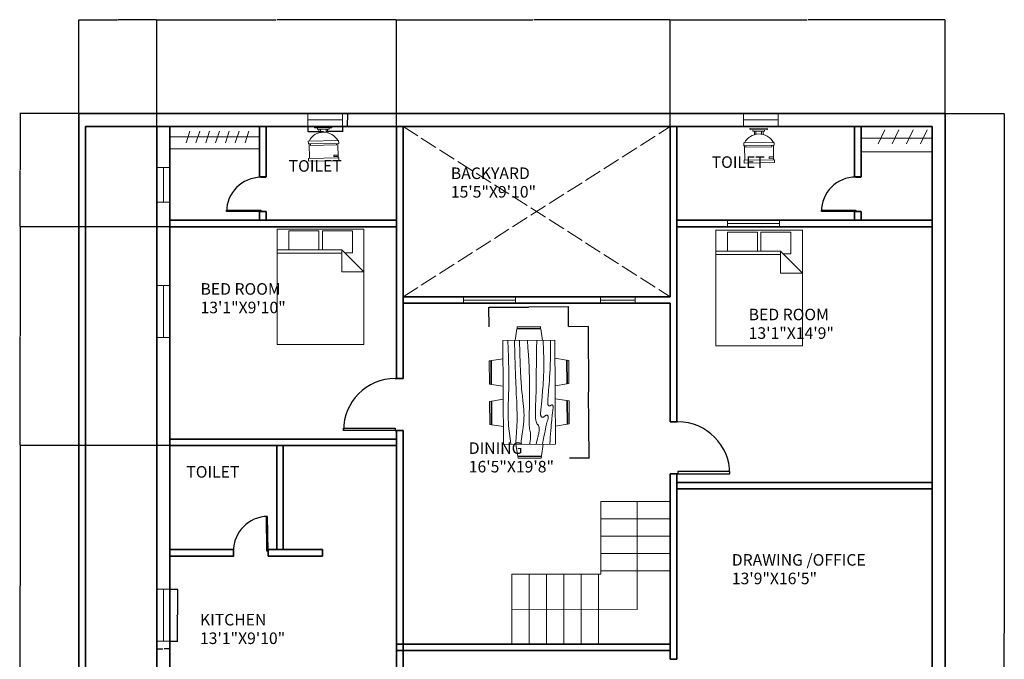
# Model space of a CAD drawing. Units: inches. Extents: x 267 to 949, y 280 to 1117.
# Tile 2 of 2: x 267 to 949, y 674 to 1117. Entities that reach past the tile are written whole.
import ezdxf

# ---------------------------------------------------------------- set-up
doc = ezdxf.new("R2010")
doc.units = ezdxf.units.IN
doc.linetypes.add('ACAD_ISO02W100', pattern=[15, 12, -3])
for name, color, linetype, lineweight in [('A-ANNO-DIMS', 2, 'Continuous', 18), ('A-AREA-IDEN', 5, 'Continuous', 18), ('A-FLOR-FIXT', 3, 'Continuous', 18), ('A-FLOR-OPEN', 3, 'ACAD_ISO02W100', 13), ('A-FURN-FIXD', 3, 'Continuous', 18), ('A-FURN-PATT', 8, 'Continuous', 13), ('DOOR', 1, 'Continuous', 25), ('FUR', 3, 'Continuous', 18), ('STAIR', 4, 'Continuous', 18), ('WALL', 7, 'Continuous', 35), ('WIN', 2, 'Continuous', 20)]:
    doc.layers.add(name, color=color, linetype=linetype, lineweight=lineweight)
doc.styles.get("Standard").update_dxf_attribs({"font": 'arial.ttf'})
doc.dimstyles.get("Standard").update_dxf_attribs({"dimtxt": 0.18, "dimasz": 0.18, "dimexe": 0.18, "dimexo": 0.0625, "dimgap": 0.09, "dimtad": 0, "dimtih": 1, "dimtoh": 1, "dimdec": 4, "dimzin": 0, "dimdsep": 46, "dimtxsty": 'Standard', "dimcen": 0.09, "dimadec": 0, "dimazin": 0, "dimtfac": 1, "dimtdec": 4, "dimtofl": 0, "dimtmove": 0, "dimatfit": 3, "dimfxl": 1, "dimtolj": 1, "dimtzin": 0, "dimarcsym": 0})

# ---------------------------------------------------------------- blocks, each defined once
blk = doc.blocks.new('*U2')
for p, q in [((0, 0), (0, -6)), ((40, 0), (40, -6))]:
    blk.add_line(p, q)
blk.add_lwpolyline([(0, 0), (0, 40), (1.75, 40), (1.75, 0)], close=True)
blk.add_arc((0, 0), 40, 0, 90)
blk = doc.blocks.new('*U3')
for p, q in [((0, 0), (0, 6)), ((40, 0), (40, 6))]:
    blk.add_line(p, q)
blk.add_lwpolyline([(0, 0), (0, -40), (1.75, -40), (1.75, 0)], close=True)
blk.add_arc((0, 0), 40, 270, 360)
blk = doc.blocks.new('*U4')
for p, q in [((0, 0), (0, 6)), ((40, 0), (40, 6))]:
    blk.add_line(p, q)
blk.add_lwpolyline([(0, 0), (0, -40), (1.75, -40), (1.75, 0)], close=True)
blk.add_arc((0, 0), 40, 270, 0)
blk = doc.blocks.new('Bed - Queen')
for p, q in [((0, -80.00003), (0, 0)), ((0, 0), (59.99999, 0)), ((59.99999, 0), (59.99999, -80.00003)), ((7.99999, -1.2), (28.79998, -1.2)), ((7.99999, -14.4), (7.99999, -1.2)), ((28.79998, -1.2), (28.79998, -14.4)), ((31.19999, -1.2), (51.99999, -1.2)), ((31.19999, -14.4), (31.19999, -1.2)), ((51.99999, -1.2), (51.99999, -16.4)), ((0, -14.4), (44.8, -14.4)), ((44.8, -16.8), (0, -16.8)), ((59.99999, -29.6), (44.8, -14.4)), ((44.8, -14.4), (44.8, -29.6)), ((51.99999, -16.4), (46.79936, -16.4)), ((44.8, -29.6), (59.99999, -29.6)), ((59.99999, -80.00003), (0, -80.00003))]:
    blk.add_line(p, q)
blk = doc.blocks.new('Dining Set - 36 x 72 in.')
for p, q in [((-22, 27.5), (-22.1562, 26.50042)), ((-22, 27.5), (-6, 27.5)), ((-5.8437, 26.49966), (-6, 27.5)), ((6, 27.5), (5.8438, 26.50042)), ((6, 27.5), (22, 27.5)), ((22.1563, 26.49966), (22, 27.5)), ((-22.2343, 26.00059), (-23.4847, 17.99762)), ((-22.2304, 26), (-5.7608, 26)), ((-5.8416, 26.5), (-22.1534, 26.5)), ((-4.5152, 17.99762), (-5.7655, 25.99926)), ((5.7657, 26.00059), (4.5153, 17.99762)), ((5.7696, 26), (22.2392, 26)), ((22.1584, 26.5), (5.8466, 26.5)), ((23.4848, 17.99762), (22.2345, 25.99926)), ((36, 18), (-36, 18)), ((-36, 18), (-36, -18)), ((36, -18), (36, 18)), ((-45.5, 8), (-44.5004, 8.15617)), ((-45.5, 8), (-45.5, -8)), ((-44.5, -8.15843), (-44.5, 8.15338)), ((-44.0006, 8.23428), (-35.9976, 9.48474)), ((-44, 8.23041), (-44, -8.23915)), ((44.0006, 8.23428), (35.9976, 9.48474)), ((44, 8.23041), (44, -8.23915)), ((44.5, -8.15843), (44.5, 8.15338)), ((45.5, 8), (44.5005, 8.15617)), ((45.5, 8), (45.5, -8)), ((-44.4997, -8.15631), (-45.5, -8)), ((-35.9976, -9.48476), (-43.9993, -8.2345)), ((35.9976, -9.48476), (43.9993, -8.2345)), ((44.4997, -8.15631), (45.5, -8)), ((-36, -18), (36, -18)), ((-22.2343, -26.0006), (-23.4847, -17.99762)), ((-4.5152, -17.99762), (-5.7655, -25.99928)), ((5.7657, -26.0006), (4.5153, -17.99762)), ((23.4848, -17.99762), (22.2345, -25.99928)), ((-22.2304, -26), (-5.7608, -26)), ((-22, -27.5), (-22.1562, -26.50044)), ((-5.8416, -26.5), (-22.1534, -26.5)), ((-5.8437, -26.49967), (-6, -27.5)), ((5.7696, -26), (22.2392, -26)), ((6, -27.5), (5.8438, -26.50044)), ((22.1584, -26.5), (5.8466, -26.5)), ((22.1563, -26.49967), (22, -27.5)), ((-22, -27.5), (-6, -27.5)), ((6, -27.5), (22, -27.5))]:
    blk.add_line(p, q)
for points in [[(-36, 15), (-31.1772, 14.97754), (-26.8079, 14.91406), (-22.8538, 14.81543), (-19.276, 14.6875), (-16.0362, 14.53613), (-13.0957, 14.36718), (-10.4159, 14.18652), (-7.9583, 14), (-5.6904, 13.81315), (-3.6035, 13.63021), (-1.6954, 13.45508), (0.0365, 13.29166), (1.5945, 13.14388), (2.9811, 13.01562), (4.1988, 12.9108), (5.25, 12.83333), (6.1393, 12.78613), (6.8802, 12.76823), (7.4883, 12.77767), (7.9792, 12.8125), (8.3685, 12.87077), (8.6719, 12.95052), (8.9049, 13.0498), (9.0833, 13.16666), (9.2205, 13.29899), (9.3216, 13.44401), (9.3895, 13.59879), (9.4271, 13.76041), (9.4373, 13.92594), (9.4232, 14.09245), (9.3875, 14.257), (9.3333, 14.41666), (9.2638, 14.56917), (9.1836, 14.71484), (9.0975, 14.85465), (9.0104, 14.98958), (8.9272, 15.1206), (8.8529, 15.2487), (8.7922, 15.37483), (8.75, 15.5), (8.7305, 15.62467), (8.7344, 15.74739), (8.7617, 15.86621), (8.8125, 15.97916), (8.8867, 16.08431), (8.9844, 16.17968), (9.1055, 16.26334), (9.25, 16.33333), (9.4189, 16.38802), (9.6172, 16.42708), (9.8506, 16.45052), (10.125, 16.45833), (10.4463, 16.45052), (10.8203, 16.42708), (11.2529, 16.38802), (11.75, 16.33333), (12.3184, 16.26318), (12.9694, 16.17838), (13.7151, 16.07991), (14.5677, 15.96875), (15.5395, 15.84586), (16.6426, 15.71224), (17.8893, 15.56884), (19.2917, 15.41666), (20.859, 15.25667), (22.5879, 15.08984), (24.4721, 14.91715), (26.5052, 14.73958), (28.6809, 14.5581), (30.9929, 14.3737), (33.4347, 14.18733), (36, 14)], [(-36, 10), (-28.9766, 10.14274), (-23.1725, 10.20442), (-18.4241, 10.19775), (-14.5677, 10.13541), (-11.4399, 10.03011), (-8.877, 9.89453), (-6.7154, 9.74137), (-4.7917, 9.58333), (-2.9698, 9.43082), (-1.2246, 9.28515), (0.4415, 9.14534), (2.026, 9.01041), (3.5266, 8.87939), (4.9408, 8.7513), (6.266, 8.62516), (7.5, 8.5), (8.6411, 8.37549), (9.6914, 8.2539), (10.6538, 8.13818), (11.5312, 8.03125), (12.3267, 7.93603), (13.043, 7.85547), (13.6831, 7.79248), (14.25, 7.75), (14.7471, 7.7303), (15.1797, 7.73307), (15.5537, 7.75732), (15.875, 7.80208), (16.1494, 7.86637), (16.3828, 7.94922), (16.5811, 8.04964), (16.75, 8.16666), (16.8944, 8.29915), (17.0143, 8.44531), (17.1089, 8.60319), (17.1771, 8.77083), (17.218, 8.94629), (17.2305, 9.1276), (17.2137, 9.31282), (17.1667, 9.5), (17.0895, 9.6875), (16.987, 9.875), (16.8649, 10.0625), (16.7292, 10.25), (16.5856, 10.4375), (16.4401, 10.625), (16.2985, 10.8125), (16.1667, 11), (16.05, 11.18733), (15.9518, 11.3737), (15.8752, 11.5581), (15.8229, 11.73958), (15.798, 11.91715), (15.8034, 12.08984), (15.842, 12.25667), (15.9167, 12.41666), (16.0295, 12.56836), (16.1784, 12.70833), (16.3605, 12.83268), (16.5729, 12.9375), (16.8127, 13.01888), (17.0768, 13.07291), (17.3625, 13.0957), (17.6667, 13.08333), (17.9894, 13.03312), (18.3418, 12.94726), (18.7382, 12.82918), (19.1927, 12.68229), (19.7195, 12.51001), (20.3327, 12.31575), (21.0465, 12.10294), (21.875, 11.875), (22.8357, 11.63354), (23.959, 11.37304), (25.2786, 11.08618), (26.8282, 10.76562), (28.6414, 10.40405), (30.752, 9.99414), (33.1936, 9.52856), (36, 9)], [(-36, 5.5), (-30.7157, 5.3348), (-26.069, 5.20963), (-21.9946, 5.11767), (-18.4271, 5.05208), (-15.3009, 5.00602), (-12.5508, 4.97265), (-10.1112, 4.94515), (-7.9167, 4.91666), (-5.909, 4.88167), (-4.0586, 4.83984), (-2.3429, 4.79215), (-0.7396, 4.73958), (0.7739, 4.6831), (2.22, 4.6237), (3.6213, 4.56233), (5, 4.5), (6.373, 4.43782), (7.7344, 4.3776), (9.0723, 4.32129), (10.375, 4.27083), (11.6309, 4.22819), (12.8281, 4.19531), (13.9551, 4.17415), (15, 4.16666), (15.954, 4.17448), (16.819, 4.19791), (17.6001, 4.23698), (18.3021, 4.29166), (18.9299, 4.36198), (19.4883, 4.44791), (19.9823, 4.54948), (20.4167, 4.66666), (20.7969, 4.79899), (21.1302, 4.94401), (21.4245, 5.09879), (21.6875, 5.26041), (21.9271, 5.42594), (22.1511, 5.59245), (22.3672, 5.757), (22.5834, 5.91666), (22.8065, 6.06868), (23.0404, 6.21093), (23.2879, 6.34147), (23.5521, 6.45833), (23.8358, 6.55957), (24.142, 6.64323), (24.4735, 6.70735), (24.8334, 6.75), (25.2235, 6.76969), (25.642, 6.76692), (26.0858, 6.74267), (26.5521, 6.69791), (27.0379, 6.63362), (27.5404, 6.55078), (28.0565, 6.45036), (28.5834, 6.33333), (29.1242, 6.19987), (29.7071, 6.04687), (30.3661, 5.87044), (31.1354, 5.66666), (32.0493, 5.43164), (33.142, 5.16146), (34.4475, 4.85221), (36, 4.5)], [(-36, -1), (-30.7915, -0.6591), (-26.0195, -0.38216), (-21.6519, -0.16284), (-17.6563, 0.00521), (-14.0005, 0.12833), (-10.6523, 0.21289), (-7.5796, 0.26522), (-4.75, 0.29166), (-2.134, 0.29793), (0.2878, 0.28711), (2.5317, 0.26163), (4.6146, 0.22396), (6.5529, 0.17651), (8.3633, 0.12174), (10.0623, 0.06209), (11.6667, 0), (13.1899, -0.06201), (14.6341, -0.1211), (15.9982, -0.17432), (17.2813, -0.21875), (18.4823, -0.25147), (19.6003, -0.26953), (20.6343, -0.27002), (21.5834, -0.25), (22.4481, -0.20768), (23.2357, -0.14584), (23.9549, -0.06836), (24.6146, 0.02083), (25.2235, 0.11784), (25.7904, 0.21875), (26.3241, 0.31966), (26.8334, 0.41666), (27.3265, 0.50618), (27.8099, 0.58593), (28.2894, 0.65397), (28.7709, 0.70833), (29.2601, 0.74707), (29.763, 0.76823), (30.2855, 0.76985), (30.8334, 0.75), (31.4088, 0.70784), (31.9994, 0.64713), (32.589, 0.57275), (33.1615, 0.48958), (33.7008, 0.4025), (34.1908, 0.3164), (34.6153, 0.23616), (34.9584, 0.16666), (35.2099, 0.11165), (35.3848, 0.07031), (35.504, 0.04069), (35.5886, 0.02083), (35.6594, 0.00879), (35.7377, 0.0026), (35.8442, 0.00032), (36, 0)], [(-36, -6.5), (-27.1843, -6.31267), (-20.084, -6.1263), (-14.469, -5.9419), (-10.1094, -5.76042), (-6.7752, -5.58285), (-4.2363, -5.41016), (-2.2629, -5.24333), (-0.625, -5.08334), (0.8708, -4.93099), (2.2715, -4.78646), (3.5872, -4.64974), (4.8281, -4.52084), (6.0046, -4.39974), (7.127, -4.28646), (8.2053, -4.18099), (9.25, -4.08334), (10.2705, -3.99382), (11.2734, -3.91407), (12.2647, -3.84603), (13.25, -3.79167), (14.2354, -3.75293), (15.2266, -3.73177), (16.2295, -3.73015), (17.25, -3.75), (18.2912, -3.79248), (19.3451, -3.85547), (20.4009, -3.93604), (21.4479, -4.03125), (22.4754, -4.13819), (23.4727, -4.25391), (24.4289, -4.37549), (25.3334, -4.5), (26.1785, -4.62492), (26.9694, -4.74935), (27.7145, -4.87281), (28.4219, -4.99479), (29.1, -5.11483), (29.7572, -5.23242), (30.4016, -5.34709), (31.0417, -5.45834), (31.6837, -5.56437), (32.3262, -5.65821), (32.9658, -5.73153), (33.599, -5.77604), (34.2224, -5.78345), (34.8327, -5.74545), (35.4264, -5.65373), (36, -5.5)], [(-36, -10), (-26.4022, -9.81299), (-18.4675, -9.62891), (-11.9839, -9.45069), (-6.7396, -9.28125), (-2.5226, -9.12354), (0.8789, -8.98047), (3.6769, -8.85498), (6.0833, -8.75), (8.2767, -8.66765), (10.3021, -8.60677), (12.1712, -8.56543), (13.8958, -8.54167), (15.4876, -8.53353), (16.9583, -8.53907), (18.3197, -8.55632), (19.5834, -8.58334), (20.7616, -8.61841), (21.8685, -8.66081), (22.9188, -8.71004), (23.9271, -8.76563), (24.9081, -8.82707), (25.8763, -8.89388), (26.8465, -8.96558), (27.8334, -9.04167), (28.8474, -9.12118), (29.8828, -9.20117), (30.93, -9.27824), (31.9792, -9.34896), (33.0205, -9.40991), (34.0443, -9.45768), (35.0407, -9.48885), (36, -9.5)], [(-36, -14.5), (-30.0881, -14.33513), (-25.0332, -14.21224), (-20.7312, -14.12647), (-17.0781, -14.07292), (-13.97, -14.04671), (-11.3027, -14.04297), (-8.9724, -14.05681), (-6.875, -14.08334), (-4.9224, -14.11833), (-3.0905, -14.16016), (-1.3709, -14.20785), (0.2448, -14.26042), (1.7647, -14.3169), (3.1973, -14.3763), (4.5507, -14.43767), (5.8333, -14.5), (7.0554, -14.5621), (8.235, -14.62175), (9.3922, -14.67652), (10.5469, -14.72396), (11.7192, -14.76164), (12.929, -14.78711), (14.1965, -14.79794), (15.5417, -14.79167), (16.9933, -14.76424), (18.6152, -14.70508), (20.4804, -14.60197), (22.6615, -14.44271), (25.2312, -14.21509), (28.2624, -13.9069), (31.8277, -13.50594), (36, -13)]]:
    blk.add_lwpolyline(points)
blk = doc.blocks.new('*U13')
for p, q in [((-10, 22), (-10, 12)), ((-10, 21), (-7, 21)), ((-7, 21), (-7, 20)), ((10, 12), (10, 22)), ((-7, 20), (-10, 20)), ((10.5, 12), (-10.5, 12)), ((-10.5, 10), (-10.5, 12)), ((10.5, 10), (-10.5, 10)), ((9, 13), (-9, 13)), ((-9, 13), (-9, 12)), ((9, 12), (9, 13)), ((10.5, 12), (10.5, 10)), ((4, 2), (-4, 2)), ((-4, 2), (-4, 1)), ((-3, 4.4065), (-3, 2)), ((-2, 2), (-2, 4.1658)), ((2, 4.1658), (2, 2)), ((3, 2), (3, 4.4065)), ((4, 1), (4, 2))]:
    blk.add_line(p, q)
for points in [[(10.5, 22), (10.5, 24), (-10.5, 24), (-10.5, 22)], [(6, 0), (6, 1), (-6, 1), (-6, 0)]]:
    blk.add_lwpolyline(points, close=True)
blk.add_arc((0, 15.3333), 11.3333, 208.0725, 331.9275)
blk = doc.blocks.new('WIN-24x9')
for p, q in [((0, 9), (0, 0)), ((24, 9), (0, 9)), ((24, 0), (24, 9)), ((0, 4.5), (24, 4.5)), ((0, 0), (24, 0))]:
    blk.add_line(p, q)
blk = doc.blocks.new('WIN-36x9')
for p, q in [((0, 36), (9, 36)), ((0, 0), (0, 36)), ((4.5, 36), (4.5, 0)), ((9, 36), (9, 0)), ((9, 0), (0, 0))]:
    blk.add_line(p, q)
blk = doc.blocks.new('WIN-36x4_5')
for p, q in [((0, 4.5), (0, 0)), ((36, 4.5), (0, 4.5)), ((0, 2.25), (36, 2.25)), ((36, 0), (36, 4.5)), ((0, 0), (36, 0))]:
    blk.add_line(p, q)
blk = doc.blocks.new('*D23')
at = {"layer": 'A-ANNO-DIMS', "color": 0, "lineweight": -2, "transparency": 16777216}
for p, q in [((466.27, 1042.96), (466.27, 1039.24)), ((466.45, 1039.42), (477.03, 1039.42)), ((490.09, 1039.42), (479.5, 1039.42)), ((490.27, 1042.96), (490.27, 1039.24))]:
    blk.add_line(p, q, dxfattribs=at)
at = {"layer": 'A-ANNO-DIMS', "color": 0, "transparency": 16777216}
for points in [[(466.45, 1039.45), (466.45, 1039.39), (466.27, 1039.42)], [(490.09, 1039.45), (490.09, 1039.39), (490.27, 1039.42)]]:
    blk.add_solid(points, dxfattribs=at)
at = {"layer": 'Defpoints', "color": 0, "transparency": 16777216}
for p in [(466.27, 1043.02), (490.27, 1043.02), (490.27, 1039.42)]:
    blk.add_point(p, dxfattribs=at)
at = {"layer": 'A-ANNO-DIMS', "color": 0, "transparency": 16777216, "insert": (478.27, 1039.42), "char_height": 0.18, "attachment_point": 5}
blk.add_mtext('\\A1;WINDOW A 24 TYP.', dxfattribs=at)
blk = doc.blocks.new('*D24')
at = {"layer": 'A-ANNO-DIMS', "color": 0, "lineweight": -2, "transparency": 16777216}
for p, q in [((490.33, 1052.02), (494.05, 1052.02)), ((493.87, 1051.84), (493.87, 1047.7)), ((493.87, 1043.2), (493.87, 1047.34)), ((490.33, 1043.02), (494.05, 1043.02))]:
    blk.add_line(p, q, dxfattribs=at)
at = {"layer": 'A-ANNO-DIMS', "color": 0, "transparency": 16777216}
for points in [[(493.84, 1051.84), (493.9, 1051.84), (493.87, 1052.02)], [(493.84, 1043.2), (493.9, 1043.2), (493.87, 1043.02)]]:
    blk.add_solid(points, dxfattribs=at)
at = {"layer": 'Defpoints', "color": 0, "transparency": 16777216}
for p in [(490.27, 1052.02), (493.87, 1052.02), (490.27, 1043.02)]:
    blk.add_point(p, dxfattribs=at)
at = {"layer": 'A-ANNO-DIMS', "color": 0, "transparency": 16777216, "insert": (493.87, 1047.52), "char_height": 0.18, "attachment_point": 5}
blk.add_mtext('\\A1;9 TYP.', dxfattribs=at)
blk = doc.blocks.new('*D25')
at = {"layer": 'A-ANNO-DIMS', "color": 0, "lineweight": -2, "transparency": 16777216}
for p, q in [((370.8, 722.58), (376.32, 722.58)), ((376.14, 722.4), (376.14, 704.77)), ((376.14, 686.76), (376.14, 704.4)), ((370.8, 686.58), (376.32, 686.58))]:
    blk.add_line(p, q, dxfattribs=at)
at = {"layer": 'A-ANNO-DIMS', "color": 0, "transparency": 16777216}
for points in [[(376.11, 722.4), (376.17, 722.4), (376.14, 722.58)], [(376.11, 686.76), (376.17, 686.76), (376.14, 686.58)]]:
    blk.add_solid(points, dxfattribs=at)
at = {"layer": 'Defpoints', "color": 0, "transparency": 16777216}
for p in [(370.74, 722.58), (376.14, 722.58), (370.74, 686.58)]:
    blk.add_point(p, dxfattribs=at)
at = {"layer": 'A-ANNO-DIMS', "color": 0, "transparency": 16777216, "insert": (376.14, 704.58), "char_height": 0.18, "attachment_point": 5}
blk.add_mtext('\\A1;WINDOW B 36 TYP.', dxfattribs=at)
blk = doc.blocks.new('*D26')
at = {"layer": 'A-ANNO-DIMS', "color": 0, "lineweight": -2, "transparency": 16777216}
for p, q in [((361.74, 686.52), (361.74, 681)), ((370.74, 686.52), (370.74, 681)), ((361.92, 681.18), (365.78, 681.18)), ((370.56, 681.18), (366.7, 681.18))]:
    blk.add_line(p, q, dxfattribs=at)
at = {"layer": 'A-ANNO-DIMS', "color": 0, "transparency": 16777216}
for points in [[(361.92, 681.21), (361.92, 681.15), (361.74, 681.18)], [(370.56, 681.21), (370.56, 681.15), (370.74, 681.18)]]:
    blk.add_solid(points, dxfattribs=at)
at = {"layer": 'Defpoints', "color": 0, "transparency": 16777216}
for p in [(361.74, 686.58), (370.74, 686.58), (370.74, 681.18)]:
    blk.add_point(p, dxfattribs=at)
at = {"layer": 'A-ANNO-DIMS', "color": 0, "transparency": 16777216, "insert": (366.24, 681.18), "char_height": 0.18, "attachment_point": 5}
blk.add_mtext('\\A1;9 TYP.', dxfattribs=at)
blk = doc.blocks.new('*D33')
at = {"layer": 'A-ANNO-DIMS', "color": 0, "lineweight": -2, "transparency": 16777216}
for p, q in [((646.88, 904.52), (660.65, 904.61)), ((660.47, 904.43), (660.78, 859.3)), ((661.09, 813.79), (660.78, 858.93)), ((647.5, 813.52), (661.27, 813.62))]:
    blk.add_line(p, q, dxfattribs=at)
at = {"layer": 'A-ANNO-DIMS', "color": 0, "transparency": 16777216}
for points in [[(660.5, 904.43), (660.44, 904.43), (660.47, 904.61)], [(661.12, 813.79), (661.06, 813.79), (661.09, 813.61)]]:
    blk.add_solid(points, dxfattribs=at)
at = {"layer": 'Defpoints', "color": 0, "transparency": 16777216}
for p in [(646.82, 904.52), (647.44, 813.52), (661.09, 813.61)]:
    blk.add_point(p, dxfattribs=at)
at = {"layer": 'A-ANNO-DIMS', "color": 0, "transparency": 16777216, "insert": (660.78, 859.11), "char_height": 0.18, "attachment_point": 5}
blk.add_mtext('\\A1;DINING SET 91', dxfattribs=at)
blk = doc.blocks.new('*D34')
at = {"layer": 'A-ANNO-DIMS', "color": 0, "lineweight": -2, "transparency": 16777216}
for p, q in [((591.82, 904.21), (591.73, 917.97)), ((591.91, 917.79), (619.01, 917.98)), ((646.55, 918.17), (619.45, 917.98)), ((646.82, 904.58), (646.73, 918.35))]:
    blk.add_line(p, q, dxfattribs=at)
at = {"layer": 'A-ANNO-DIMS', "color": 0, "transparency": 16777216}
for points in [[(591.91, 917.82), (591.91, 917.76), (591.73, 917.79)], [(646.55, 918.2), (646.55, 918.14), (646.73, 918.17)]]:
    blk.add_solid(points, dxfattribs=at)
at = {"layer": 'Defpoints', "color": 0, "transparency": 16777216}
for p in [(646.73, 918.17), (591.82, 904.14), (646.82, 904.52)]:
    blk.add_point(p, dxfattribs=at)
at = {"layer": 'A-ANNO-DIMS', "color": 0, "transparency": 16777216, "insert": (619.23, 917.98), "char_height": 0.18, "attachment_point": 5}
blk.add_mtext('\\A1;55', dxfattribs=at)
blk = doc.blocks.new('*D36')
at = {"layer": 'A-ANNO-DIMS', "color": 0, "lineweight": -2, "transparency": 16777216}
for p, q in [((907.8, 1052.02), (948.62, 1052.02)), ((948.44, 1051.84), (948.44, 692.2)), ((948.44, 332.2), (948.44, 691.84)), ((907.8, 332.02), (948.62, 332.02))]:
    blk.add_line(p, q, dxfattribs=at)
at = {"layer": 'A-ANNO-DIMS', "color": 0, "transparency": 16777216}
for points in [[(948.41, 1051.84), (948.47, 1051.84), (948.44, 1052.02)], [(948.41, 332.2), (948.47, 332.2), (948.44, 332.02)]]:
    blk.add_solid(points, dxfattribs=at)
at = {"layer": 'Defpoints', "color": 0, "transparency": 16777216}
for p in [(907.74, 1052.02), (948.44, 1052.02), (907.74, 332.02)]:
    blk.add_point(p, dxfattribs=at)
at = {"layer": 'A-ANNO-DIMS', "color": 0, "transparency": 16777216, "insert": (948.44, 692.02), "char_height": 0.18, "attachment_point": 5}
blk.add_mtext('\\A1;720', dxfattribs=at)
blk = doc.blocks.new('*D37')
at = {"layer": 'A-ANNO-DIMS', "color": 0, "lineweight": -2, "transparency": 16777216}
for p, q in [((307.74, 1052.08), (307.74, 1116.93)), ((307.92, 1116.75), (334.52, 1116.75)), ((361.56, 1116.75), (334.96, 1116.75)), ((361.74, 1043.08), (361.74, 1116.93))]:
    blk.add_line(p, q, dxfattribs=at)
at = {"layer": 'A-ANNO-DIMS', "color": 0, "transparency": 16777216}
for points in [[(307.92, 1116.78), (307.92, 1116.72), (307.74, 1116.75)], [(361.56, 1116.78), (361.56, 1116.72), (361.74, 1116.75)]]:
    blk.add_solid(points, dxfattribs=at)
at = {"layer": 'Defpoints', "color": 0, "transparency": 16777216}
for p in [(361.74, 1116.75), (307.74, 1052.02), (361.74, 1043.02)]:
    blk.add_point(p, dxfattribs=at)
at = {"layer": 'A-ANNO-DIMS', "color": 0, "transparency": 16777216, "insert": (334.74, 1116.75), "char_height": 0.18, "attachment_point": 5}
blk.add_mtext('\\A1;54', dxfattribs=at)
blk = doc.blocks.new('*D38')
at = {"layer": 'A-ANNO-DIMS', "color": 0, "lineweight": -2, "transparency": 16777216}
for p, q in [((361.74, 1043.08), (361.74, 1116.93)), ((361.92, 1116.75), (444.46, 1116.75)), ((527.56, 1116.75), (445.02, 1116.75)), ((527.74, 1043.08), (527.74, 1116.93))]:
    blk.add_line(p, q, dxfattribs=at)
at = {"layer": 'A-ANNO-DIMS', "color": 0, "transparency": 16777216}
for points in [[(361.92, 1116.78), (361.92, 1116.72), (361.74, 1116.75)], [(527.56, 1116.78), (527.56, 1116.72), (527.74, 1116.75)]]:
    blk.add_solid(points, dxfattribs=at)
at = {"layer": 'Defpoints', "color": 0, "transparency": 16777216}
for p in [(527.74, 1116.75), (361.74, 1043.02), (527.74, 1043.02)]:
    blk.add_point(p, dxfattribs=at)
at = {"layer": 'A-ANNO-DIMS', "color": 0, "transparency": 16777216, "insert": (444.74, 1116.75), "char_height": 0.18, "attachment_point": 5}
blk.add_mtext('\\A1;166', dxfattribs=at)
blk = doc.blocks.new('*D39')
at = {"layer": 'A-ANNO-DIMS', "color": 0, "lineweight": -2, "transparency": 16777216}
for p, q in [((527.74, 1043.08), (527.74, 1116.93)), ((527.92, 1116.75), (622.1, 1116.75)), ((717.06, 1116.75), (622.88, 1116.75)), ((717.24, 1043.08), (717.24, 1116.93))]:
    blk.add_line(p, q, dxfattribs=at)
at = {"layer": 'A-ANNO-DIMS', "color": 0, "transparency": 16777216}
for points in [[(527.92, 1116.78), (527.92, 1116.72), (527.74, 1116.75)], [(717.06, 1116.78), (717.06, 1116.72), (717.24, 1116.75)]]:
    blk.add_solid(points, dxfattribs=at)
at = {"layer": 'Defpoints', "color": 0, "transparency": 16777216}
for p in [(717.24, 1116.75), (527.74, 1043.02), (717.24, 1043.02)]:
    blk.add_point(p, dxfattribs=at)
at = {"layer": 'A-ANNO-DIMS', "color": 0, "transparency": 16777216, "insert": (622.49, 1116.75), "char_height": 0.18, "attachment_point": 5}
blk.add_mtext('\\A1;189.5', dxfattribs=at)
blk = doc.blocks.new('*D40')
at = {"layer": 'A-ANNO-DIMS', "color": 0, "lineweight": -2, "transparency": 16777216}
for p, q in [((717.24, 1043.08), (717.24, 1116.93)), ((717.42, 1116.75), (812.1, 1116.75)), ((907.56, 1116.75), (812.88, 1116.75)), ((907.74, 1052.08), (907.74, 1116.93))]:
    blk.add_line(p, q, dxfattribs=at)
at = {"layer": 'A-ANNO-DIMS', "color": 0, "transparency": 16777216}
for points in [[(717.42, 1116.78), (717.42, 1116.72), (717.24, 1116.75)], [(907.56, 1116.78), (907.56, 1116.72), (907.74, 1116.75)]]:
    blk.add_solid(points, dxfattribs=at)
at = {"layer": 'Defpoints', "color": 0, "transparency": 16777216}
for p in [(907.74, 1116.75), (907.74, 1052.02), (717.24, 1043.02)]:
    blk.add_point(p, dxfattribs=at)
at = {"layer": 'A-ANNO-DIMS', "color": 0, "transparency": 16777216, "insert": (812.49, 1116.75), "char_height": 0.18, "attachment_point": 5}
blk.add_mtext('\\A1;190.5', dxfattribs=at)
blk = doc.blocks.new('*D44')
at = {"layer": 'A-ANNO-DIMS', "color": 0, "lineweight": -2, "transparency": 16777216}
for p, q in [((370.68, 822.02), (266.86, 822.02)), ((267.04, 821.84), (267.04, 724.95)), ((267.04, 627.7), (267.04, 724.59)), ((370.68, 627.52), (266.86, 627.52))]:
    blk.add_line(p, q, dxfattribs=at)
at = {"layer": 'A-ANNO-DIMS', "color": 0, "transparency": 16777216}
for points in [[(267.01, 821.84), (267.07, 821.84), (267.04, 822.02)], [(267.01, 627.7), (267.07, 627.7), (267.04, 627.52)]]:
    blk.add_solid(points, dxfattribs=at)
at = {"layer": 'Defpoints', "color": 0, "transparency": 16777216}
for p in [(267.04, 822.02), (370.74, 822.02), (370.74, 627.52)]:
    blk.add_point(p, dxfattribs=at)
at = {"layer": 'A-ANNO-DIMS', "color": 0, "transparency": 16777216, "insert": (267.04, 724.77), "char_height": 0.18, "attachment_point": 5}
blk.add_mtext('\\A1;194.5', dxfattribs=at)
blk = doc.blocks.new('*D45')
at = {"layer": 'A-ANNO-DIMS', "color": 0, "lineweight": -2, "transparency": 16777216}
for p, q in [((370.68, 973.52), (266.86, 973.52)), ((267.04, 973.34), (267.04, 897.95)), ((267.04, 822.2), (267.04, 897.59)), ((370.68, 822.02), (266.86, 822.02))]:
    blk.add_line(p, q, dxfattribs=at)
at = {"layer": 'A-ANNO-DIMS', "color": 0, "transparency": 16777216}
for points in [[(267.01, 973.34), (267.07, 973.34), (267.04, 973.52)], [(267.01, 822.2), (267.07, 822.2), (267.04, 822.02)]]:
    blk.add_solid(points, dxfattribs=at)
at = {"layer": 'Defpoints', "color": 0, "transparency": 16777216}
for p in [(267.04, 973.52), (370.74, 973.52), (370.74, 822.02)]:
    blk.add_point(p, dxfattribs=at)
at = {"layer": 'A-ANNO-DIMS', "color": 0, "transparency": 16777216, "insert": (267.04, 897.77), "char_height": 0.18, "attachment_point": 5}
blk.add_mtext('\\A1;151.5', dxfattribs=at)
blk = doc.blocks.new('*D46')
at = {"layer": 'A-ANNO-DIMS', "color": 0, "lineweight": -2, "transparency": 16777216}
for p, q in [((307.68, 1052.02), (266.86, 1052.02)), ((267.04, 1051.84), (267.04, 1012.95)), ((267.04, 973.7), (267.04, 1012.59)), ((370.68, 973.52), (266.86, 973.52))]:
    blk.add_line(p, q, dxfattribs=at)
at = {"layer": 'A-ANNO-DIMS', "color": 0, "transparency": 16777216}
for points in [[(267.01, 1051.84), (267.07, 1051.84), (267.04, 1052.02)], [(267.01, 973.7), (267.07, 973.7), (267.04, 973.52)]]:
    blk.add_solid(points, dxfattribs=at)
at = {"layer": 'Defpoints', "color": 0, "transparency": 16777216}
for p in [(267.04, 1052.02), (307.74, 1052.02), (370.74, 973.52)]:
    blk.add_point(p, dxfattribs=at)
at = {"layer": 'A-ANNO-DIMS', "color": 0, "transparency": 16777216, "insert": (267.04, 1012.77), "char_height": 0.18, "attachment_point": 5}
blk.add_mtext('\\A1;78.5', dxfattribs=at)

msp = doc.modelspace()

# ---------------------------------------------------------------- hatches: boundary and pattern name
at = {"layer": 'A-FURN-PATT'}
h = msp.add_hatch(dxfattribs=at)
h.set_pattern_fill('ANSI31', color=256, scale=2.03235, angle=26.364, style=0)
h.paths.add_polyline_path([(376.3839, 1031.5713), (426.553, 1031.5713), (429.2744, 1039.6412), (379.1053, 1039.6412)])
h = msp.add_hatch(dxfattribs=at)
h.set_pattern_fill('ANSI31', color=256, scale=2.76973, angle=18.76, style=0)
h.paths.add_polyline_path([(854.055, 1031.0587), (892.5213, 1031.0587), (897.2103, 1040.571), (858.744, 1040.571)])

# ---------------------------------------------------------------- linework, layer by layer
at = {"layer": 'A-FLOR-OPEN'}
for p, q in [((532.2409, 1043.0219), (717.2409, 925.0219)), ((532.2409, 925.0219), (717.2409, 1043.0219))]:
    msp.add_line(p, q, dxfattribs=at)
at = {"layer": 'A-FURN-FIXD'}
for p, q in [((370.7409, 1035.8705), (432.8683, 1035.8705)), ((849.4625, 1034.8875), (898.7409, 1034.8875)), ((370.7409, 1027.518), (432.8683, 1027.518)), ((849.4625, 1025.5219), (898.7409, 1025.5219))]:
    msp.add_line(p, q, dxfattribs=at)
at = {"layer": 'STAIR'}
for p, q in [((717.2409, 783.3872), (669.2409, 783.3872)), ((669.2409, 783.3872), (669.2409, 733.0485)), ((694.3317, 708.5918), (694.3317, 783.3872)), ((717.2409, 771.3872), (669.2409, 771.3872)), ((717.2409, 759.3872), (669.2409, 759.3872)), ((717.2409, 747.3872), (669.2409, 747.3872)), ((669.2409, 733.0485), (607.6359, 733.0485)), ((607.6359, 733.0485), (607.6359, 684.5219)), ((619.6359, 733.0485), (619.6359, 684.5219)), ((631.6359, 733.0485), (631.6359, 684.5219)), ((643.6359, 733.0485), (643.6359, 684.5219)), ((655.6359, 733.0485), (655.6359, 684.5219)), ((667.6359, 733.0485), (667.6359, 684.5219)), ((717.2409, 735.3872), (669.2409, 735.3872)), ((607.6359, 708.7852), (694.3317, 708.5918))]:
    msp.add_line(p, q, dxfattribs=at)
at = {"layer": 'WALL'}
for p, q in [((307.7409, 1052.0219), (907.7409, 1052.0219)), ((307.7409, 1052.0219), (307.7409, 332.0219)), ((907.7409, 1052.0219), (907.7409, 332.0219)), ((312.2409, 1043.0219), (898.7409, 1043.0219)), ((312.2409, 1043.0219), (312.2409, 336.5219)), ((361.7409, 1043.0219), (361.7409, 399.5219)), ((361.7409, 1043.0219), (361.7409, 399.5219)), ((361.7409, 1043.0219), (361.7409, 399.5219)), ((370.7409, 1043.0219), (370.7409, 408.5219)), ((432.8683, 1043.0219), (432.8683, 1008.0219)), ((437.3683, 1043.0219), (437.3683, 1008.0219)), ((527.7409, 1043.0219), (527.7409, 868.5219)), ((532.2409, 1043.0219), (532.2409, 868.5219)), ((717.2409, 1043.0219), (717.2409, 925.0219)), ((721.7409, 1043.0219), (721.7409, 838.5219)), ((844.9625, 1043.0219), (844.9625, 1008.0219)), ((849.4625, 1043.0219), (849.4625, 1008.0219)), ((898.7409, 1043.0219), (898.7409, 336.5219)), ((432.8683, 1008.0219), (437.3683, 1008.0219)), ((844.9625, 1008.0219), (849.4625, 1008.0219)), ((432.8683, 978.0219), (432.8683, 984.0219)), ((432.8683, 984.0219), (437.3683, 984.0219)), ((432.8683, 984.0219), (432.8683, 978.0219)), ((437.3683, 984.0219), (437.3683, 978.0219)), ((844.9625, 978.0219), (844.9625, 984.0219)), ((844.9625, 984.0219), (849.4625, 984.0219)), ((844.9625, 984.0219), (844.9625, 978.0219)), ((849.4625, 984.0219), (849.4625, 978.0219)), ((370.7409, 978.0219), (527.7409, 978.0219)), ((721.7409, 978.0219), (898.7409, 978.0219)), ((370.7409, 973.5219), (527.7409, 973.5219)), ((721.7409, 973.5219), (898.7409, 973.5219)), ((532.2409, 925.0219), (717.2409, 925.0219)), ((532.2409, 920.5219), (717.2409, 920.5219)), ((717.2409, 920.5219), (717.2409, 838.5219)), ((527.7409, 868.5219), (532.2409, 868.5219)), ((527.7409, 826.5219), (527.7409, 832.5219)), ((527.7409, 832.5219), (532.2409, 832.5219)), ((527.7409, 832.5219), (527.7409, 551.0219)), ((532.2409, 832.5219), (532.2409, 492.0219)), ((721.7409, 838.5219), (717.2409, 838.5219)), ((370.7409, 826.5219), (527.7409, 826.5219)), ((370.7409, 822.0219), (527.7409, 822.0219)), ((444.7409, 822.0219), (444.7409, 750.0219)), ((449.2409, 822.0219), (449.2409, 750.0219)), ((721.7409, 802.5219), (717.2409, 802.5219)), ((717.2409, 802.5219), (717.2409, 674.0219)), ((721.7409, 796.5219), (721.7409, 802.5219)), ((721.7409, 802.5219), (721.7409, 674.0219)), ((721.7409, 796.5219), (898.7409, 796.5219)), ((721.7409, 792.0219), (898.7409, 792.0219)), ((370.7409, 750.0219), (414.7409, 750.0219)), ((370.7409, 745.5219), (414.7409, 745.5219)), ((414.7409, 750.0219), (414.7409, 745.5219)), ((444.7409, 750.0219), (438.7409, 750.0219)), ((438.7409, 750.0219), (438.7409, 745.5219)), ((438.7409, 750.0219), (476.4951, 750.0219)), ((438.7409, 745.5219), (476.4951, 745.5219)), ((476.4951, 750.0219), (476.4951, 745.5219)), ((527.7409, 684.5219), (717.2409, 684.5219)), ((527.7409, 680.0219), (717.2409, 680.0219)), ((717.2409, 680.0219), (717.2409, 674.0219)), ((717.2409, 674.0219), (721.7409, 674.0219))]:
    msp.add_line(p, q, dxfattribs=at)
at = {"layer": 'WIN'}
for p, q in [((466.265, 1052.0219), (466.265, 1043.0219)), ((668.9891, 925.0219), (668.9891, 920.5219)), ((692.9891, 925.0219), (668.9891, 925.0219)), ((668.9891, 922.7719), (692.9891, 922.7719)), ((692.9891, 920.5219), (692.9891, 925.0219)), ((668.9891, 920.5219), (692.9891, 920.5219))]:
    msp.add_line(p, q, dxfattribs=at)

# ---------------------------------------------------------------- block references
at = {"layer": 'A-FLOR-FIXT', "rotation": 180.9809891052875}
for p in [(476.9536, 1043.0561), (778.5139, 1041.7793)]:
    msp.add_blockref('*U13', p, dxfattribs=at)
at = {"layer": 'DOOR'}
for name, p, xscale, yscale, zscale, rotation in [('*U2', (433.803, 984.0219), 0.594212098592789, 0.594212098592789, 0.594212098592789, 90), ('*U2', (845.8705, 984.0219), 0.5986589731677388, 0.5986589731677388, 0.5986589731677388, 90), ('*U2', (526.8527, 832.5219), 0.898029023570897, 0.898029023570897, 0.898029023570897, 90), ('*U3', (722.6291, 802.5219), 0.898029023570897, 0.898029023570897, 0.898029023570897, 90), ('*U4', (438.7055, 749.1051), 0.5972278222085773, 0.5972278222085773, 0.5972278222085773, 180.5661466738159)]:
    msp.add_blockref(name, p, dxfattribs=dict(at, xscale=xscale, yscale=yscale, zscale=zscale, rotation=rotation))
at = {"layer": 'FUR'}
for p in [(445.143, 971.9683), (748.8987, 971.0937)]:
    msp.add_blockref('Bed - Queen', p, dxfattribs=at)
at = {"layer": 'FUR', "rotation": 270.3912682758113}
msp.add_blockref('Dining Set - 36 x 72 in.', (619.631, 858.8317), dxfattribs=at)
at = {"layer": 'WIN'}
for name, p in [('WIN-24x9', (466.265, 1043.022)), ('WIN-24x9', (768.0624, 1043.022)), ('WIN-36x4_5', (756.899, 973.522)), ('WIN-36x9', (361.741, 896.89)), ('WIN-36x4_5', (574.1061, 920.522)), ('WIN-36x9', (361.741, 686.5818))]:
    msp.add_blockref(name, p, dxfattribs=at)
at = {"layer": 'WIN', "rotation": 270.000000000001}
msp.add_blockref('WIN-24x9', (361.741, 1014.5931), dxfattribs=at)

# ---------------------------------------------------------------- texts
at = {"layer": 'A-AREA-IDEN'}
for s, p in [('TOILET', (453.0199, 1011.6762)), ('TOILET', (745.9912, 1014.3179)), ('BACKYARD', (565.3295, 1006.597)), ('15\'5"X9\'10"', (565.3295, 993.7457)), ('BED ROOM', (391.9608, 926.4929)), ('13\'1"X9\'10"', (391.9608, 913.6416)), ('BED ROOM', (771.6042, 908.7872)), ('13\'1"X14\'9"', (771.6042, 895.9359)), ('DINING', (577.7464, 816.2735)), ('16\'5"X19\'8"', (577.7464, 803.4222)), ('TOILET', (382.1481, 799.8276)), ('DRAWING /OFFICE', (759.9255, 738.8686)), ('13\'9"X16\'5"', (759.9255, 726.0173)), ('KITCHEN', (391.5785, 697.4473)), ('13\'1"X9\'10"', (391.5785, 684.596))]:
    msp.add_text(s, height=8, dxfattribs=at).set_placement(p)

# ---------------------------------------------------------------- dimensions: what is measured, and where the dimension line sits
at = {"layer": 'A-ANNO-DIMS'}
for base, p1, p2, override, picture, middle in [((361.7409, 1116.7513), (307.7409, 1052.0219), (361.7409, 1043.0219), {"dimdec": 0, "dimlfac": 1, "dimrnd": 0, "dimzin": 0, "dimdsep": 46, "dimlunit": 2}, '*D37', (334.7409, 1116.7513)), ((527.7409, 1116.7513), (361.7409, 1043.0219), (527.7409, 1043.0219), {"dimdec": 0, "dimlfac": 1, "dimrnd": 0, "dimzin": 0, "dimdsep": 46, "dimlunit": 2}, '*D38', (444.7409, 1116.7513)), ((717.2409, 1116.7513), (527.7409, 1043.0219), (717.2409, 1043.0219), {"dimdec": 1, "dimlfac": 1, "dimrnd": 0, "dimzin": 0, "dimdsep": 46, "dimlunit": 2}, '*D39', (622.4909, 1116.7513)), ((907.7409, 1116.7513), (717.2409, 1043.0219), (907.7409, 1052.0219), {"dimdec": 1, "dimlfac": 1, "dimrnd": 0, "dimzin": 0, "dimdsep": 46, "dimlunit": 2}, '*D40', (812.4909, 1116.7513))]:
    dim = msp.add_linear_dim(base=base, p1=p1, p2=p2, dimstyle='Standard', override=override, dxfattribs=at)
    dim.commit()
    dim.dimension.update_dxf_attribs({"geometry": picture, "text_midpoint": middle})
for base, p1, p2, angle, override, picture, middle in [((267.0409, 1052.0219), (370.7409, 973.5219), (307.7409, 1052.0219), 90, {"dimdec": 1, "dimlfac": 1, "dimrnd": 0, "dimzin": 0, "dimdsep": 46, "dimlunit": 2}, '*D46', (267.0409, 1012.7719)), ((948.4409, 1052.0219), (907.7409, 332.0219), (907.7409, 1052.0219), 90, {"dimdec": 0, "dimlfac": 1, "dimrnd": 0, "dimzin": 0, "dimdsep": 46, "dimlunit": 2}, '*D36', (948.4409, 692.0219)), ((267.0409, 973.5219), (370.7409, 822.0219), (370.7409, 973.5219), 90, {"dimdec": 1, "dimlfac": 1, "dimrnd": 0, "dimzin": 0, "dimdsep": 46, "dimlunit": 2}, '*D45', (267.0409, 897.7719)), ((646.7264, 918.1681), (591.8209, 904.1429), (646.8196, 904.5184), 0.3912683, {"dimdec": 0, "dimlfac": 1, "dimrnd": 0, "dimzin": 0, "dimdsep": 46, "dimlunit": 2}, '*D34', (619.2271, 917.9803)), ((267.0409, 822.0219), (370.7409, 627.5219), (370.7409, 822.0219), 90, {"dimdec": 1, "dimlfac": 1, "dimrnd": 0, "dimzin": 0, "dimdsep": 46, "dimlunit": 2}, '*D44', (267.0409, 724.7719))]:
    dim = msp.add_linear_dim(base=base, p1=p1, p2=p2, angle=angle, dimstyle='Standard', override=override, dxfattribs=at)
    dim.commit()
    dim.dimension.update_dxf_attribs({"geometry": picture, "text_midpoint": middle})
for base, p1, p2, angle, text, picture, middle in [((493.865, 1052.0219), (490.265, 1043.0219), (490.265, 1052.0219), 90, '<> TYP.', '*D24', (493.865, 1047.5219)), ((661.0907, 813.6138), (646.8196, 904.5184), (647.4411, 813.5206), 270.3912683, 'DINING SET <>', '*D33', (660.78, 859.1127)), ((376.1409, 722.5819), (370.7409, 686.5819), (370.7409, 722.5819), 90, 'WINDOW B <> TYP.', '*D25', (376.1409, 704.5819))]:
    dim = msp.add_linear_dim(base=base, p1=p1, p2=p2, angle=angle, text=text, dimstyle='Standard', override={"dimdec": 0, "dimlfac": 1, "dimrnd": 0, "dimzin": 0, "dimdsep": 46, "dimlunit": 2}, dxfattribs=at)
    dim.commit()
    dim.dimension.update_dxf_attribs({"geometry": picture, "text_midpoint": middle})
for base, p1, p2, text, picture, middle in [((490.265, 1039.4219), (466.265, 1043.0219), (490.265, 1043.0219), 'WINDOW A <> TYP.', '*D23', (478.265, 1039.4219)), ((370.7409, 681.1819), (361.7409, 686.5819), (370.7409, 686.5819), '<> TYP.', '*D26', (366.2409, 681.1819))]:
    dim = msp.add_linear_dim(base=base, p1=p1, p2=p2, text=text, dimstyle='Standard', override={"dimdec": 0, "dimlfac": 1, "dimrnd": 0, "dimzin": 0, "dimdsep": 46, "dimlunit": 2}, dxfattribs=at)
    dim.commit()
    dim.dimension.update_dxf_attribs({"geometry": picture, "text_midpoint": middle})

doc.saveas('drawing.dxf')
